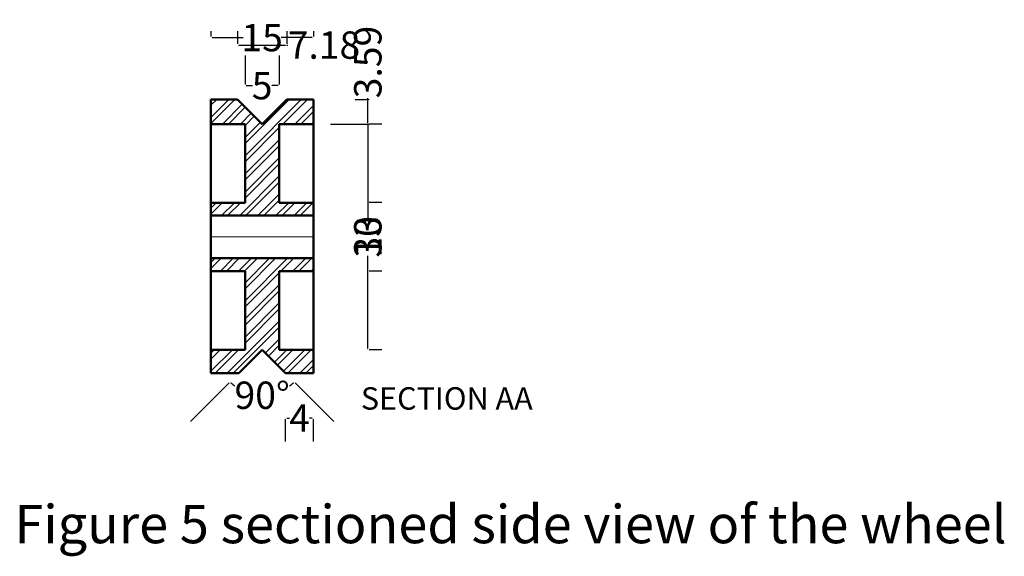
# Model space of a CAD drawing. Units: millimetres. Extents: x 1183 to 1513, y 471 to 941.
# Tile 2 of 3: x 1367 to 1511, y 636 to 714. Entities that reach past the tile are written whole.
import ezdxf

# ---------------------------------------------------------------- set-up
doc = ezdxf.new("R2010")
doc.units = ezdxf.units.MM
doc.header["$LTSCALE"] = 1.4
doc.header["$MEASUREMENT"] = 0
doc.linetypes.add('CENTER', pattern=[50.8, 31.75, -6.35, 6.35, -6.35])
for name, color, linetype, lineweight in [('M-CNTR', 1, 'CENTER', 18), ('M-DIMS', 2, 'Continuous', 25), ('M-HATC', 8, 'Continuous', 18), ('M-OUTL', 7, 'Continuous', 50), ('M-TEXT', 3, 'Continuous', 25)]:
    doc.layers.add(name, color=color, linetype=linetype, lineweight=lineweight)
doc.styles.get("Standard").update_dxf_attribs({"font": 'arial.ttf'})
doc.dimstyles.get("Standard").update_dxf_attribs({"dimtxt": 4, "dimasz": 0.18, "dimexe": 0.18, "dimexo": 10, "dimgap": 0.09, "dimtad": 0, "dimdec": 0, "dimzin": 0, "dimdsep": 46, "dimtxsty": 'Standard', "dimcen": 0.09, "dimadec": 0, "dimazin": 0, "dimtfac": 1, "dimtdec": 0, "dimtofl": 0, "dimtmove": 0, "dimatfit": 3, "dimfxl": 1, "dimtolj": 1, "dimtzin": 0, "dimarcsym": 0})

# ---------------------------------------------------------------- blocks, each defined once
blk = doc.blocks.new('*D26')
at = {"layer": 'Defpoints', "color": 0, "lineweight": 140, "ltscale": 0.13, "transparency": 16777216}
for p in [(1402.66, 666.04), (1402.66, 666.04), (1399.25, 662.63), (1406.07, 662.63), (1400.94, 659.61)]:
    blk.add_point(p, dxfattribs=at)
at = {"layer": 'M-DIMS', "color": 0, "lineweight": -2, "ltscale": 0.13, "transparency": 16777216}
for p, q in [((1392.18, 655.56), (1397.83, 661.21)), ((1413.14, 655.56), (1407.49, 661.21))]:
    blk.add_line(p, q, dxfattribs=at)
for start, end in [(226.5498, 232.9074), (307.0926, 313.4502)]:
    blk.add_arc((1402.66, 666.04), 6.65, start, end, dxfattribs=at)
at = {"layer": 'M-DIMS', "color": 0, "lineweight": 140, "ltscale": 0.13, "transparency": 16777216}
for points in [[(1398.06, 661.19), (1398.1, 661.23), (1397.95, 661.33)], [(1407.22, 661.23), (1407.26, 661.19), (1407.37, 661.33)]]:
    blk.add_solid(points, dxfattribs=at)
at = {"layer": 'M-DIMS', "color": 0, "ltscale": 0.13, "transparency": 16777216, "insert": (1402.66, 659.38), "char_height": 4, "attachment_point": 5}
blk.add_mtext('\\A1;90°', dxfattribs=at)
blk = doc.blocks.new('*D27')
at = {"layer": 'Defpoints', "color": 0, "lineweight": 140, "ltscale": 0.13, "transparency": 16777216}
for p in [(1405.16, 704.65), (1400.16, 699.04), (1405.16, 699.04)]:
    blk.add_point(p, dxfattribs=at)
at = {"layer": 'M-DIMS', "color": 0, "lineweight": -2, "ltscale": 0.13, "transparency": 16777216}
for p, q in [((1400.16, 709.04), (1400.16, 704.83)), ((1405.16, 709.04), (1405.16, 704.83)), ((1400.34, 704.65), (1401.24, 704.65)), ((1404.98, 704.65), (1404.08, 704.65))]:
    blk.add_line(p, q, dxfattribs=at)
at = {"layer": 'M-DIMS', "color": 0, "lineweight": 140, "ltscale": 0.13, "transparency": 16777216}
for points in [[(1400.34, 704.68), (1400.34, 704.62), (1400.16, 704.65)], [(1404.98, 704.68), (1404.98, 704.62), (1405.16, 704.65)]]:
    blk.add_solid(points, dxfattribs=at)
at = {"layer": 'M-DIMS', "color": 0, "ltscale": 0.13, "transparency": 16777216, "insert": (1402.66, 704.65), "char_height": 4, "attachment_point": 5}
blk.add_mtext('\\A1;5', dxfattribs=at)
blk = doc.blocks.new('*D28')
at = {"layer": 'Defpoints', "color": 0, "lineweight": 140, "ltscale": 0.13, "transparency": 16777216}
for p in [(1410.16, 711.67), (1395.16, 702.63), (1410.16, 702.63)]:
    blk.add_point(p, dxfattribs=at)
at = {"layer": 'M-DIMS', "color": 0, "lineweight": -2, "ltscale": 0.13, "transparency": 16777216}
for p, q in [((1395.16, 712.63), (1395.16, 711.85)), ((1410.16, 712.63), (1410.16, 711.85)), ((1395.34, 711.67), (1399.88, 711.67)), ((1409.98, 711.67), (1405.44, 711.67))]:
    blk.add_line(p, q, dxfattribs=at)
at = {"layer": 'M-DIMS', "color": 0, "lineweight": 140, "ltscale": 0.13, "transparency": 16777216}
for points in [[(1395.34, 711.7), (1395.34, 711.64), (1395.16, 711.67)], [(1409.98, 711.7), (1409.98, 711.64), (1410.16, 711.67)]]:
    blk.add_solid(points, dxfattribs=at)
at = {"layer": 'M-DIMS', "color": 0, "ltscale": 0.13, "transparency": 16777216, "insert": (1402.66, 711.67), "char_height": 4, "attachment_point": 5}
blk.add_mtext('\\A1;15', dxfattribs=at)
blk = doc.blocks.new('*D29')
at = {"layer": 'Defpoints', "color": 0, "lineweight": 140, "ltscale": 0.13, "transparency": 16777216}
for p in [(1406.07, 662.63), (1410.16, 662.63), (1410.16, 656.05)]:
    blk.add_point(p, dxfattribs=at)
at = {"layer": 'M-DIMS', "color": 0, "lineweight": -2, "ltscale": 0.13, "transparency": 16777216}
for p, q in [((1406.07, 652.63), (1406.07, 655.87)), ((1406.25, 656.05), (1406.64, 656.05)), ((1409.98, 656.05), (1409.59, 656.05)), ((1410.16, 652.63), (1410.16, 655.87))]:
    blk.add_line(p, q, dxfattribs=at)
at = {"layer": 'M-DIMS', "color": 0, "lineweight": 140, "ltscale": 0.13, "transparency": 16777216}
for points in [[(1406.25, 656.08), (1406.25, 656.02), (1406.07, 656.05)], [(1409.98, 656.08), (1409.98, 656.02), (1410.16, 656.05)]]:
    blk.add_solid(points, dxfattribs=at)
at = {"layer": 'M-DIMS', "color": 0, "ltscale": 0.13, "transparency": 16777216, "insert": (1408.12, 656.05), "char_height": 4, "attachment_point": 5}
blk.add_mtext('\\A1;4', dxfattribs=at)
blk = doc.blocks.new('*D48')
at = {"layer": 'Defpoints', "color": 0, "lineweight": 140, "ltscale": 1.4, "transparency": 16777216}
for p in [(1410.16, 699.04), (1410.16, 666.04), (1418.11, 666.04)]:
    blk.add_point(p, dxfattribs=at)
at = {"layer": 'M-DIMS', "color": 0, "lineweight": -2, "ltscale": 1.4, "transparency": 16777216}
for p, q in [((1418.11, 698.86), (1418.11, 685.49)), ((1420.16, 699.04), (1418.29, 699.04)), ((1418.11, 666.22), (1418.11, 679.59)), ((1420.16, 666.04), (1418.29, 666.04))]:
    blk.add_line(p, q, dxfattribs=at)
at = {"layer": 'M-DIMS', "color": 0, "lineweight": 140, "ltscale": 1.4, "transparency": 16777216}
for points in [[(1418.08, 698.86), (1418.14, 698.86), (1418.11, 699.04)], [(1418.08, 666.22), (1418.14, 666.22), (1418.11, 666.04)]]:
    blk.add_solid(points, dxfattribs=at)
at = {"layer": 'M-DIMS', "color": 0, "ltscale": 1.4, "transparency": 16777216, "insert": (1418.11, 682.54), "char_height": 4, "attachment_point": 5, "rotation": 90}
blk.add_mtext('\\A1;33', dxfattribs=at)
blk = doc.blocks.new('*D49')
at = {"layer": 'Defpoints', "color": 0, "lineweight": 140, "ltscale": 1.4, "transparency": 16777216}
for p in [(1410.16, 687.54), (1410.16, 677.54), (1418.11, 677.54)]:
    blk.add_point(p, dxfattribs=at)
at = {"layer": 'M-DIMS', "color": 0, "lineweight": -2, "ltscale": 1.4, "transparency": 16777216}
for p, q in [((1418.11, 687.36), (1418.11, 685.3)), ((1420.16, 687.54), (1418.29, 687.54)), ((1418.11, 677.72), (1418.11, 679.78)), ((1420.16, 677.54), (1418.29, 677.54))]:
    blk.add_line(p, q, dxfattribs=at)
at = {"layer": 'M-DIMS', "color": 0, "lineweight": 140, "ltscale": 1.4, "transparency": 16777216}
for points in [[(1418.08, 687.36), (1418.14, 687.36), (1418.11, 687.54)], [(1418.08, 677.72), (1418.14, 677.72), (1418.11, 677.54)]]:
    blk.add_solid(points, dxfattribs=at)
at = {"layer": 'M-DIMS', "color": 0, "ltscale": 1.4, "transparency": 16777216, "insert": (1418.11, 682.54), "char_height": 4, "attachment_point": 5, "rotation": 90}
blk.add_mtext('\\A1;10', dxfattribs=at)
blk = doc.blocks.new('*D50')
at = {"layer": 'Defpoints', "color": 0, "lineweight": 140, "ltscale": 1.4, "transparency": 16777216}
for p in [(1406.25, 702.63), (1418.11, 702.63), (1402.66, 699.04)]:
    blk.add_point(p, dxfattribs=at)
at = {"layer": 'M-DIMS', "color": 0, "lineweight": -2, "ltscale": 1.4, "transparency": 16777216}
for p, q in [((1416.25, 702.63), (1418.29, 702.63)), ((1418.11, 702.63), (1418.11, 702.81)), ((1418.11, 699.22), (1418.11, 702.45)), ((1412.66, 699.04), (1418.29, 699.04))]:
    blk.add_line(p, q, dxfattribs=at)
at = {"layer": 'M-DIMS', "color": 0, "lineweight": 140, "ltscale": 1.4, "transparency": 16777216}
for points in [[(1418.08, 702.45), (1418.14, 702.45), (1418.11, 702.63)], [(1418.08, 699.22), (1418.14, 699.22), (1418.11, 699.04)]]:
    blk.add_solid(points, dxfattribs=at)
at = {"layer": 'M-DIMS', "color": 0, "ltscale": 1.4, "transparency": 16777216, "insert": (1418.11, 708.1), "char_height": 4, "attachment_point": 5, "rotation": 90}
blk.add_mtext('\\A1;3.59', dxfattribs=at)
blk = doc.blocks.new('*D51')
at = {"layer": 'Defpoints', "color": 0, "lineweight": 140, "ltscale": 1.4, "transparency": 16777216}
for p in [(1406.25, 710.58), (1399.07, 702.63), (1406.25, 702.63)]:
    blk.add_point(p, dxfattribs=at)
at = {"layer": 'M-DIMS', "color": 0, "lineweight": -2, "ltscale": 1.4, "transparency": 16777216}
for p, q in [((1399.07, 712.63), (1399.07, 710.76)), ((1406.25, 712.63), (1406.25, 710.76)), ((1399.25, 710.58), (1406.07, 710.58)), ((1406.25, 710.58), (1406.43, 710.58))]:
    blk.add_line(p, q, dxfattribs=at)
at = {"layer": 'M-DIMS', "color": 0, "lineweight": 140, "ltscale": 1.4, "transparency": 16777216}
for points in [[(1399.25, 710.61), (1399.25, 710.55), (1399.07, 710.58)], [(1406.07, 710.61), (1406.07, 710.55), (1406.25, 710.58)]]:
    blk.add_solid(points, dxfattribs=at)
at = {"layer": 'M-DIMS', "color": 0, "ltscale": 1.4, "transparency": 16777216, "insert": (1411.7, 710.58), "char_height": 4, "attachment_point": 5}
blk.add_mtext('\\A1;7.18', dxfattribs=at)

msp = doc.modelspace()

# ---------------------------------------------------------------- hatches: boundary and pattern name
at = {"layer": 'M-HATC', "ltscale": 0.13}
h = msp.add_hatch(dxfattribs=at)
h.set_pattern_fill('ANSI32', color=256, scale=5)
h.set_pattern_definition([(45, (-411.4872, -205.0805), (-1.3258252, 1.3258252), []), (45, (-410.6033, -205.0805), (-1.3258252, 1.3258252), [])])
h.paths.add_polyline_path([(1405.1606, 677.5388), (1410.1606, 677.5388), (1410.1606, 679.4138), (1395.1606, 679.4138), (1395.1606, 677.5388), (1400.1606, 677.5388), (1400.1606, 666.0388), (1395.1606, 666.0388), (1395.1606, 662.6288), (1399.2506, 662.6288), (1402.6606, 666.0388), (1406.0706, 662.6288), (1410.1606, 662.6288), (1410.1606, 666.0388), (1405.1606, 666.0388)])
h.paths.add_polyline_path([(1405.1606, 699.0388), (1410.1606, 699.0388), (1410.1606, 702.6288), (1406.2506, 702.6288), (1402.6606, 699.0388), (1399.0706, 702.6288), (1395.1606, 702.6288), (1395.1606, 699.0388), (1400.1606, 699.0388), (1400.1606, 687.5388), (1395.1606, 687.5388), (1395.1606, 685.6638), (1410.1606, 685.6638), (1410.1606, 687.5388), (1405.1606, 687.5388)])

# ---------------------------------------------------------------- linework, layer by layer
at = {"layer": 'M-CNTR', "ltscale": 2}
msp.add_line((1395.1606, 682.5388), (1410.1606, 682.5388), dxfattribs=at)
at = {"layer": 'M-OUTL', "ltscale": 0.13}
for p, q in [((1395.1606, 702.6288), (1399.0706, 702.6288)), ((1395.1606, 662.6288), (1395.1606, 702.6288)), ((1402.6606, 699.0388), (1399.0706, 702.6288)), ((1402.6606, 699.0388), (1406.2506, 702.6288)), ((1406.2506, 702.6288), (1410.1606, 702.6288)), ((1410.1606, 662.6288), (1410.1606, 702.6288)), ((1395.1606, 699.0388), (1400.1606, 699.0388)), ((1405.1606, 699.0388), (1410.1606, 699.0388)), ((1395.1606, 666.0388), (1400.1606, 666.0388)), ((1402.6606, 666.0388), (1399.2506, 662.6288)), ((1402.6606, 666.0388), (1406.0706, 662.6288)), ((1405.1606, 666.0388), (1410.1606, 666.0388)), ((1395.1606, 662.6288), (1399.2506, 662.6288)), ((1406.0706, 662.6288), (1410.1606, 662.6288))]:
    msp.add_line(p, q, dxfattribs=at)
at = {"layer": 'M-OUTL', "ltscale": 2}
for p, q in [((1400.1606, 699.0388), (1400.1606, 687.5388)), ((1405.1606, 699.0388), (1405.1606, 687.5388)), ((1395.1606, 687.5388), (1400.1606, 687.5388)), ((1405.1606, 687.5388), (1410.1606, 687.5388)), ((1395.1606, 685.6638), (1410.1606, 685.6638)), ((1395.1606, 679.4138), (1410.1606, 679.4138)), ((1395.1606, 677.5388), (1400.1606, 677.5388)), ((1400.1606, 677.5388), (1400.1606, 666.0388)), ((1405.1606, 677.5388), (1405.1606, 666.0388)), ((1405.1606, 677.5388), (1410.1606, 677.5388))]:
    msp.add_line(p, q, dxfattribs=at)

# ---------------------------------------------------------------- texts
at = {"layer": 'M-TEXT', "ltscale": 0.13}
for s, height, p in [('SECTION AA', 3.2763, (1417.0907, 657.2763)), ('Figure 5 sectioned side view of the wheel ', 5.601941, (1366.4507, 637.7405))]:
    msp.add_text(s, height=height, dxfattribs=at).set_placement(p)

# ---------------------------------------------------------------- dimensions: what is measured, and where the dimension line sits
at = {"layer": 'M-DIMS', "ltscale": 0.13}
for base, p1, p2, picture, middle in [((1410.1606, 711.669), (1395.1606, 702.6288), (1410.1606, 702.6288), '*D28', (1402.6606, 711.669)), ((1405.1606, 704.6517), (1400.1606, 699.0388), (1405.1606, 699.0388), '*D27', (1402.6606, 704.6517)), ((1410.1606, 656.0512), (1406.0706, 662.6288), (1410.1606, 662.6288), '*D29', (1408.1156, 656.0512))]:
    dim = msp.add_linear_dim(base=base, p1=p1, p2=p2, dimstyle='Standard', override={"dimclrd": 0, "dimclre": 0, "dimclrt": 0}, dxfattribs=at)
    dim.commit()
    dim.dimension.update_dxf_attribs({"geometry": picture, "text_midpoint": middle})
at = {"layer": 'M-DIMS', "ltscale": 1.4}
dim = msp.add_linear_dim(base=(1406.2506, 710.5788), p1=(1399.0706, 702.6288), p2=(1406.2506, 702.6288), dimstyle='Standard', override={"dimdec": 2, "dimlfac": 1, "dimrnd": 0, "dimzin": 0, "dimdsep": 46, "dimlunit": 2}, dxfattribs=at)
dim.commit()
dim.dimension.update_dxf_attribs({"geometry": '*D51', "text_midpoint": (1411.7034, 710.5788)})
for base, p1, p2, override, picture, middle in [((1418.1106, 702.6288), (1402.6606, 699.0388), (1406.2506, 702.6288), {"dimdec": 2, "dimlfac": 1, "dimrnd": 0, "dimzin": 0, "dimdsep": 46, "dimlunit": 2}, '*D50', (1418.1106, 708.0966)), ((1418.1106, 666.0388), (1410.1606, 699.0388), (1410.1606, 666.0388), {"dimdec": 0, "dimlfac": 1, "dimrnd": 0, "dimzin": 0, "dimdsep": 46, "dimlunit": 2}, '*D48', (1418.1106, 682.5388)), ((1418.1106, 677.5388), (1410.1606, 687.5388), (1410.1606, 677.5388), {"dimdec": 0, "dimlfac": 1, "dimrnd": 0, "dimzin": 0, "dimdsep": 46, "dimlunit": 2}, '*D49', (1418.1106, 682.5388))]:
    dim = msp.add_linear_dim(base=base, p1=p1, p2=p2, angle=90, dimstyle='Standard', override=override, dxfattribs=at)
    dim.commit()
    dim.dimension.update_dxf_attribs({"geometry": picture, "text_midpoint": middle})
at = {"layer": 'M-DIMS', "ltscale": 0.13}
dim = msp.add_angular_dim_2l(base=(1400.9382, 659.6106), line1=((1402.6606, 666.0388), (1406.0706, 662.6288)), line2=((1402.6606, 666.0388), (1399.2506, 662.6288)), dimstyle='Standard', override={"dimclrd": 0, "dimclre": 0, "dimclrt": 0}, dxfattribs=at)
dim.commit()
dim.dimension.update_dxf_attribs({"geometry": '*D26', "text_midpoint": (1402.6606, 659.3839)})

doc.saveas('drawing.dxf')
